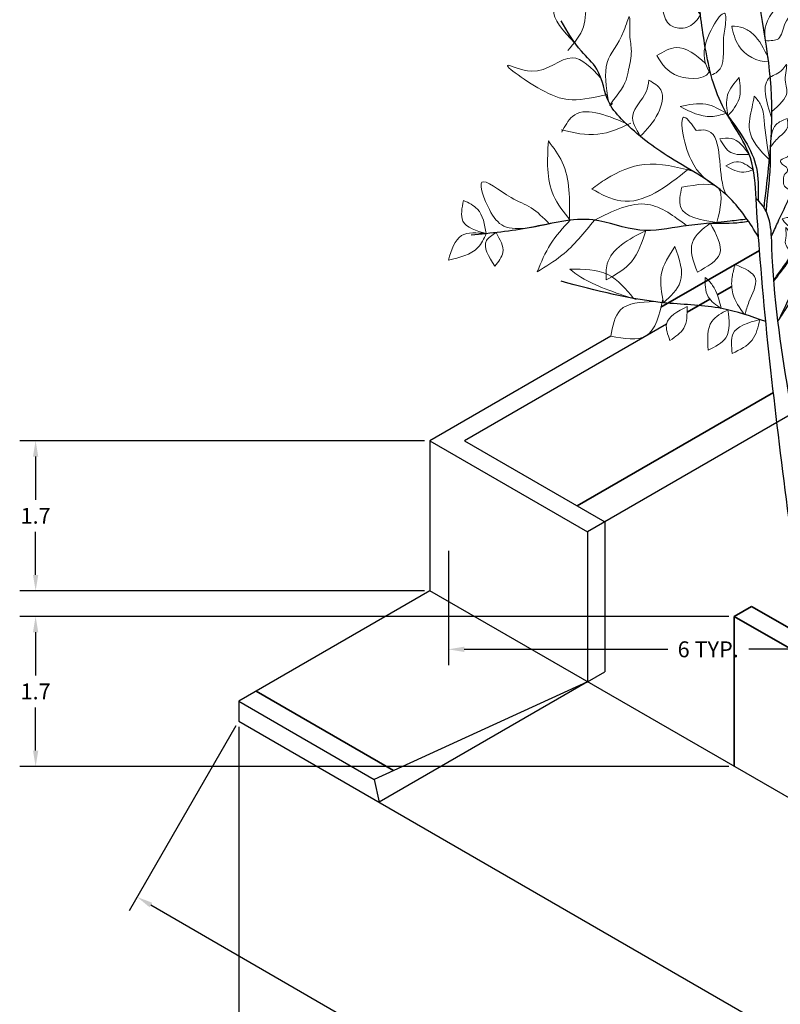
# Model space of a CAD drawing. Units: metres. Extents: x 12735 to 25554, y 20954 to 41989.
# Tile 2 of 15: x 12735.36 to 12743.97, y 20963.53 to 20974.68. Entities that reach past the tile are written whole.
import ezdxf

# ---------------------------------------------------------------- set-up
doc = ezdxf.new("R2010")
doc.units = ezdxf.units.M
doc.layers.get('Defpoints').update_dxf_attribs({"lineweight": 13})
for name, color, linetype, lineweight in [('A-ANNO-DIMS', 2, 'Continuous', 18), ('A-ELEV', 7, 'Continuous', 35), ('C-SITE', 8, 'Continuous', 25), ('TREES', 72, 'Continuous', 18)]:
    doc.layers.add(name, color=color, linetype=linetype, lineweight=lineweight)
doc.layers.add('STEM', color=32, linetype='Continuous')
doc.styles.get("Standard").update_dxf_attribs({"font": 'arial.ttf'})
doc.dimstyles.get("Standard").update_dxf_attribs({"dimtxt": 0.18, "dimasz": 0.18, "dimexe": 0.18, "dimexo": 0.0625, "dimgap": 0.09, "dimtad": 0, "dimtih": 1, "dimtoh": 1, "dimdec": 4, "dimzin": 0, "dimdsep": 46, "dimtxsty": 'Standard', "dimcen": 0.09, "dimadec": 0, "dimazin": 0, "dimtfac": 1, "dimtdec": 4, "dimtofl": 0, "dimtmove": 0, "dimatfit": 3, "dimfxl": 1, "dimtolj": 1, "dimtzin": 0, "dimarcsym": 0})

# ---------------------------------------------------------------- blocks, each defined once
blk = doc.blocks.new('TREES')
blk.add_line((12743.7, 20972.648), (12743.7, 20972.648))
at = {"layer": 'STEM'}
for points, knots in [([(12743.791, 20972.546), (12743.793, 20972.564), (12743.795, 20972.582), (12743.797, 20972.6), (12743.801, 20972.637), (12743.806, 20972.674), (12743.81, 20972.711), (12743.845, 20973.018), (12743.938, 20973.826), (12743.743, 20974.806), (12743.607, 20975.634), (12743.413, 20975.893), (12743.333, 20975.999)], [-0.164913, -0.164913, -0.164913, -0.164913, -0.110972, -0.110972, -0.110972, 0, 0, 0, 0.920963, 2.426088, 2.990404, 3.384799, 3.384799, 3.384799, 3.384799]), ([(12743.7, 20972.648), (12743.691, 20972.807), (12743.671, 20973.194), (12743.257, 20973.699), (12743.111, 20974.379), (12743.038, 20974.998), (12742.993, 20975.377), (12742.974, 20975.54)], [0, 0, 0, 0, 0.469346, 1.137622, 1.869488, 2.521439, 3.013071, 3.013071, 3.013071, 3.013071]), ([(12743.874, 20972.227), (12743.898, 20972.277), (12743.921, 20972.328), (12743.945, 20972.378), (12744.022, 20972.541), (12744.105, 20972.717), (12744.205, 20972.963), (12744.312, 20973.088), (12744.183, 20973.501), (12744.667, 20973.973), (12744.707, 20974.64), (12744.896, 20975.012), (12744.823, 20975.434), (12744.85, 20975.23), (12744.867, 20975.1)], [-0.166951, -0.166951, -0.166951, -0.166951, 0, 0, 0, 0.539768, 0.582066, 0.798222, 0.98781, 1.7696, 2.524754, 2.899414, 3.105113, 3.460848, 3.460848, 3.460848, 3.460848]), ([(12743.728, 20972.218), (12743.63, 20972.372), (12743.383, 20972.76), (12742.753, 20973.07), (12742.291, 20973.419), (12741.984, 20973.759), (12741.959, 20974.098), (12741.675, 20974.346), (12741.563, 20974.543), (12741.494, 20974.663)], [0, 0, 0, 0, 0.542161, 1.359078, 2.03444, 2.290187, 2.703676, 2.968549, 3.382864, 3.382864, 3.382864, 3.382864]), ([(12743.967, 20971.294), (12743.987, 20971.335), (12744.006, 20971.376), (12744.026, 20971.417), (12744.057, 20971.483), (12744.088, 20971.549), (12744.119, 20971.615), (12744.196, 20971.778), (12744.279, 20971.954), (12744.378, 20972.2), (12744.486, 20972.325), (12744.357, 20972.738), (12744.836, 20973.215), (12744.895, 20973.862), (12745.051, 20974.269), (12745.045, 20974.62), (12744.834, 20974.67), (12744.7, 20974.701)], [-0.355099, -0.355099, -0.355099, -0.355099, -0.218492, -0.218492, -0.218492, 0, 0, 0, 0.539768, 0.582066, 0.798222, 0.98781, 1.7696, 2.524754, 2.899414, 3.105113, 3.460848, 3.460848, 3.460848, 3.460848]), ([(12744.175, 20971.633), (12744.383, 20971.767), (12744.692, 20971.967), (12745.149, 20972.305), (12745.828, 20972.463), (12745.606, 20973.185), (12745.967, 20973.583), (12745.99, 20973.882), (12746.002, 20974.029)], [0, 0, 0, 0, 0.736164, 1.094646, 1.754618, 2.392389, 2.840214, 3.27091, 3.27091, 3.27091, 3.27091]), ([(12743.381, 20973.588), (12743.52, 20973.4), (12743.728, 20973.118), (12743.725, 20972.776), (12743.724, 20972.661), (12743.724, 20972.661), (12743.724, 20972.661), (12743.724, 20972.661), (12743.724, 20972.65), (12743.724, 20972.639), (12743.724, 20972.627)], [0, 0, 0, 0, 0.673099, 1.009429, 1.009429, 1.009429, 1.009429, 1.009429, 1.009429, 1.043412, 1.043412, 1.043412, 1.043412]), ([(12743.814, 20972.505), (12743.817, 20972.531), (12743.819, 20972.556), (12743.822, 20972.581), (12743.827, 20972.63), (12743.832, 20972.679), (12743.838, 20972.727), (12743.847, 20972.813), (12743.865, 20972.982), (12743.864, 20973.152), (12743.864, 20973.236)], [-0.2227932, -0.2227932, -0.2227932, -0.2227932, -0.1464713, -0.1464713, -0.1464713, 0, 0, 0, 0.2578951, 0.5103882, 0.5103882, 0.5103882, 0.5103882]), ([(12743.902, 20971.717), (12743.93, 20971.754), (12743.959, 20971.791), (12743.988, 20971.829), (12743.988, 20971.829), (12743.988, 20971.829), (12743.988, 20971.829), (12744.096, 20971.973), (12744.236, 20972.16), (12744.082, 20972.476), (12744.347, 20972.598), (12744.368, 20972.766), (12744.376, 20972.837)], [-0.129757, -0.129757, -0.129757, -0.129757, 0, 0, 0, 0, 0, 0, 0.485118, 0.62751, 0.913144, 1.120766, 1.120766, 1.120766, 1.120766]), ([(12744.111, 20968.725), (12743.967, 20969.837), (12743.799, 20971.142), (12743.712, 20972.453), (12743.7, 20972.648)], [0, 0, 0, 0, 3.359203, 3.944548, 3.944548, 3.944548, 3.944548]), ([(12744.332, 20968.825), (12744.189, 20969.936), (12743.871, 20971.161), (12743.872, 20972.51), (12743.7, 20972.648)], [0, 0, 0, 0, 3.359203, 3.972384, 3.972384, 3.972384, 3.972384]), ([(12743.597, 20972.418), (12743.533, 20972.41), (12743.292, 20972.379), (12742.889, 20972.351), (12742.364, 20972.241), (12741.803, 20972.489), (12741.157, 20972.302), (12740.698, 20972.258), (12740.474, 20972.237)], [0, 0, 0, 0, 0.193148, 0.727923, 1.218416, 1.762371, 2.471743, 3.152626, 3.152626, 3.152626, 3.152626]), ([(12743.181, 20972.372), (12743.296, 20972.37), (12743.441, 20972.368), (12743.583, 20972.39), (12743.613, 20972.395)], [0, 0, 0, 0, 0.3435042, 0.4329772, 0.4329772, 0.4329772, 0.4329772]), ([(12743.948, 20971.264), (12743.975, 20971.305), (12744.002, 20971.345), (12744.029, 20971.386), (12744.029, 20971.386), (12744.029, 20971.386), (12744.029, 20971.386), (12744.129, 20971.55), (12744.289, 20971.812), (12744.368, 20972.107), (12744.398, 20972.218)], [-0.148605, -0.148605, -0.148605, -0.148605, 0, 0, 0, 0, 0, 0, 0.572176, 0.914425, 0.914425, 0.914425, 0.914425]), ([(12743.901, 20971.729), (12743.929, 20971.768), (12743.958, 20971.808), (12743.986, 20971.847), (12743.986, 20971.847), (12743.986, 20971.847), (12743.986, 20971.847), (12744.02, 20971.892), (12744.062, 20971.951), (12744.099, 20972.014), (12744.107, 20972.028)], [-0.1467707, -0.1467707, -0.1467707, -0.1467707, 0, 0, 0, 0, 0, 0, 0.1684242, 0.2179474, 0.2179474, 0.2179474, 0.2179474]), ([(12743.81, 20971.258), (12743.646, 20971.316), (12743.283, 20971.443), (12742.486, 20971.453), (12741.888, 20971.61), (12741.494, 20971.714)], [0, 0, 0, 0, 0.519056, 1.146346, 2.366016, 2.366016, 2.366016, 2.366016])]:
    blk.add_open_spline(points, degree=3, knots=knots, dxfattribs=at)
blk.add_open_spline([(12744.644, 20971.941), (12744.672, 20971.961), (12744.701, 20971.98), (12744.73, 20972)], degree=3, dxfattribs=at)
at = {"layer": 'TREES'}
for points, knots in [([(12743.584, 20975.586), (12743.37, 20975.718), (12743.075, 20975.9), (12743.022, 20976.725), (12743.333, 20976.097), (12743.574, 20975.612)], [0, 0, 0, 0, 0.724771, 1.002271, 1.932196, 1.932196, 1.932196, 1.932196]), ([(12743.021, 20975.14), (12743.019, 20975.277), (12743.016, 20975.483), (12742.921, 20975.662), (12742.889, 20975.721)], [0, 0, 0, 0, 0.4023849, 0.6031293, 0.6031293, 0.6031293, 0.6031293]), ([(12743.021, 20975.14), (12742.985, 20975.224), (12742.928, 20975.356), (12742.766, 20975.539), (12742.854, 20975.638), (12742.901, 20975.69)], [0, 0, 0, 0, 0.2845416, 0.4465287, 0.6279758, 0.6279758, 0.6279758, 0.6279758]), ([(12743.718, 20974.979), (12743.671, 20975.164), (12743.598, 20975.454), (12743.323, 20975.534), (12743.223, 20975.563)], [0, 0, 0, 0, 0.519429, 0.8155501, 0.8155501, 0.8155501, 0.8155501]), ([(12743.223, 20975.563), (12743.266, 20975.448), (12743.36, 20975.195), (12743.592, 20975.055), (12743.718, 20974.979)], [0, 0, 0, 0, 0.3595778, 0.7860105, 0.7860105, 0.7860105, 0.7860105]), ([(12743.737, 20974.871), (12743.729, 20975.055), (12743.718, 20975.333), (12743.914, 20975.516), (12743.981, 20975.578)], [0, 0, 0, 0, 0.5134638, 0.7779111, 0.7779111, 0.7779111, 0.7779111]), ([(12743.737, 20974.871), (12743.801, 20974.971), (12743.939, 20975.186), (12743.966, 20975.441), (12743.981, 20975.578)], [0, 0, 0, 0, 0.351068, 0.7565079, 0.7565079, 0.7565079, 0.7565079]), ([(12741.648, 20974.411), (12741.519, 20974.547), (12741.281, 20974.798), (12741.642, 20974.995), (12741.673, 20975.511), (12741.684, 20975.149), (12741.787, 20975.033), (12741.768, 20974.824), (12741.781, 20974.575), (12741.641, 20974.411), (12741.569, 20974.326)], [0, 0, 0, 0, 0.446457, 0.821839, 1.096823, 1.294203, 1.491123, 1.594729, 1.894892, 2.216107, 2.216107, 2.216107, 2.216107]), ([(12743.031, 20975.058), (12743.048, 20975.139), (12743.077, 20975.281), (12743.184, 20975.377), (12743.231, 20975.418)], [0, 0, 0, 0, 0.2398723, 0.4207027, 0.4207027, 0.4207027, 0.4207027]), ([(12743.037, 20975.007), (12743.075, 20975.058), (12743.166, 20975.181), (12743.207, 20975.33), (12743.231, 20975.418)], [0, 0, 0, 0, 0.1895117, 0.457602, 0.457602, 0.457602, 0.457602]), ([(12744.796, 20974.806), (12744.757, 20974.909), (12744.688, 20975.088), (12744.514, 20975.28), (12744.523, 20975.414), (12744.526, 20975.464)], [0, 0, 0, 0, 0.3323117, 0.5782809, 0.7232611, 0.7232611, 0.7232611, 0.7232611]), ([(12744.805, 20974.813), (12744.804, 20974.918), (12744.803, 20975.076), (12744.822, 20975.37), (12744.643, 20975.427), (12744.526, 20975.464)], [0, 0, 0, 0, 0.3224266, 0.4885617, 0.8037384, 0.8037384, 0.8037384, 0.8037384]), ([(12743.07, 20974.733), (12742.98, 20974.863), (12742.848, 20975.053), (12742.433, 20975.446), (12742.649, 20974.915), (12742.651, 20974.573), (12742.961, 20974.576), (12743.034, 20974.678), (12743.071, 20974.73)], [0, 0, 0, 0, 0.54832, 0.799685, 1.166614, 1.565159, 1.742127, 1.925713, 1.925713, 1.925713, 1.925713]), ([(12744.796, 20974.806), (12744.882, 20974.878), (12745.017, 20974.992), (12745.211, 20975.15), (12745.228, 20975.277), (12745.236, 20975.337)], [0, 0, 0, 0, 0.3416822, 0.5370609, 0.7122352, 0.7122352, 0.7122352, 0.7122352]), ([(12744.839, 20974.951), (12744.859, 20975.055), (12744.903, 20975.272), (12745.122, 20975.315), (12745.236, 20975.337)], [0, 0, 0, 0, 0.2913456, 0.6064398, 0.6064398, 0.6064398, 0.6064398]), ([(12743.814, 20974.4), (12743.798, 20974.494), (12743.764, 20974.693), (12744.115, 20975.006), (12744.156, 20974.79), (12744.01, 20974.677), (12743.989, 20974.434), (12743.864, 20974.438), (12743.809, 20974.439)], [0, 0, 0, 0, 0.311146, 0.650746, 0.669061, 0.940573, 1.125337, 1.270427, 1.270427, 1.270427, 1.270427]), ([(12743.191, 20974.047), (12743.14, 20974.139), (12743.026, 20974.346), (12743.367, 20974.877), (12743.354, 20974.597), (12743.309, 20974.413), (12743.358, 20974.125), (12743.218, 20974.059), (12743.191, 20974.047)], [0, 0, 0, 0, 0.337622, 0.758697, 0.837919, 1.040495, 1.406258, 1.489574, 1.489574, 1.489574, 1.489574]), ([(12742.028, 20973.754), (12742.003, 20973.912), (12741.953, 20974.218), (12742.174, 20974.414), (12742.283, 20974.81), (12742.258, 20974.48), (12742.304, 20974.323), (12742.246, 20974.069), (12742.227, 20973.932), (12742.006, 20973.671), (12742.066, 20973.72), (12742.075, 20973.727)], [0, 0, 0, 0, 0.436736, 0.842969, 1.012738, 1.21393, 1.403734, 1.613178, 1.897283, 2.067562, 2.097274, 2.097274, 2.097274, 2.097274]), ([(12744.509, 20973.941), (12744.486, 20974.093), (12744.451, 20974.322), (12744.425, 20974.623), (12744.504, 20974.731), (12744.534, 20974.773)], [0, 0, 0, 0, 0.4681587, 0.7056034, 0.8580265, 0.8580265, 0.8580265, 0.8580265]), ([(12744.534, 20974.773), (12744.556, 20974.698), (12744.634, 20974.425), (12744.562, 20974.144), (12744.509, 20973.941)], [0, 0, 0, 0, 0.2327329, 0.8431329, 0.8431329, 0.8431329, 0.8431329]), ([(12744.554, 20973.975), (12744.669, 20974.016), (12744.893, 20974.094), (12745.019, 20974.421), (12745.06, 20974.624), (12745.08, 20974.72)], [0, 0, 0, 0, 0.348929, 0.678298, 0.9763146, 0.9763146, 0.9763146, 0.9763146]), ([(12743.835, 20974.249), (12743.789, 20974.346), (12743.724, 20974.484), (12743.556, 20974.594), (12743.468, 20974.601), (12743.424, 20974.604)], [0, 0, 0, 0, 0.3158223, 0.4463774, 0.5774617, 0.5774617, 0.5774617, 0.5774617]), ([(12743.424, 20974.604), (12743.442, 20974.527), (12743.487, 20974.324), (12743.715, 20974.191), (12743.841, 20974.206), (12743.841, 20974.206)], [0, 0, 0, 0, 0.2361186, 0.6165307, 0.6167763, 0.6167763, 0.6167763, 0.6167763]), ([(12744.618, 20974.118), (12744.717, 20974.268), (12744.844, 20974.462), (12745.022, 20974.606), (12745.062, 20974.638)], [0, 0, 0, 0, 0.5333846, 0.686651, 0.686651, 0.686651, 0.686651]), ([(12744.97, 20974.043), (12744.931, 20974.146), (12744.862, 20974.325), (12744.688, 20974.517), (12744.697, 20974.651), (12744.7, 20974.701)], [0, 0, 0, 0, 0.3323117, 0.5782809, 0.7232611, 0.7232611, 0.7232611, 0.7232611]), ([(12745.957, 20973.706), (12745.908, 20973.835), (12745.798, 20974.123), (12745.864, 20974.427), (12745.9, 20974.594)], [0, 0, 0, 0, 0.4051126, 0.906838, 0.906838, 0.906838, 0.906838]), ([(12745.9, 20974.594), (12745.955, 20974.471), (12746.037, 20974.287), (12746.01, 20974.092), (12746.002, 20974.029)], [0, 0, 0, 0, 0.3943838, 0.5836156, 0.5836156, 0.5836156, 0.5836156]), ([(12744.97, 20974.043), (12745.056, 20974.115), (12745.191, 20974.229), (12745.385, 20974.387), (12745.402, 20974.514), (12745.41, 20974.574)], [0, 0, 0, 0, 0.3416822, 0.5370609, 0.7122352, 0.7122352, 0.7122352, 0.7122352]), ([(12745.013, 20974.188), (12745.033, 20974.292), (12745.077, 20974.509), (12745.296, 20974.552), (12745.41, 20974.574)], [0, 0, 0, 0, 0.2913456, 0.6064398, 0.6064398, 0.6064398, 0.6064398]), ([(12743.128, 20974.182), (12743.019, 20974.275), (12742.841, 20974.427), (12742.65, 20974.313), (12742.577, 20974.27)], [0, 0, 0, 0, 0.3785086, 0.6144536, 0.6144536, 0.6144536, 0.6144536]), ([(12742.577, 20974.27), (12742.635, 20974.174), (12742.755, 20973.977), (12743.187, 20974.003), (12743.173, 20974.131), (12743.172, 20974.137)], [0, 0, 0, 0, 0.3386751, 0.6999446, 0.7185805, 0.7185805, 0.7185805, 0.7185805]), ([(12745.785, 20973.361), (12745.68, 20973.449), (12745.404, 20973.684), (12745.451, 20974.057), (12745.481, 20974.288)], [0, 0, 0, 0, 0.391493, 1.034106, 1.034106, 1.034106, 1.034106]), ([(12745.481, 20974.288), (12745.577, 20974.138), (12745.76, 20973.855), (12745.777, 20973.519), (12745.785, 20973.361)], [0, 0, 0, 0, 0.5245256, 0.9915723, 0.9915723, 0.9915723, 0.9915723]), ([(12741.943, 20974.016), (12741.835, 20974.13), (12741.594, 20974.382), (12741.272, 20973.991), (12740.687, 20974.27), (12741.289, 20973.836), (12741.63, 20973.742), (12741.878, 20973.799), (12742.016, 20973.831)], [0, 0, 0, 0, 0.397812, 0.88569, 1.156328, 1.66735, 1.991498, 2.394837, 2.394837, 2.394837, 2.394837]), ([(12743.879, 20973.555), (12743.816, 20973.752), (12743.731, 20974.021), (12743.982, 20974.067), (12744.068, 20974.224), (12744.006, 20973.984), (12744.093, 20973.824), (12743.961, 20973.709), (12743.879, 20973.638)], [0, 0, 0, 0, 0.469961, 0.638827, 0.705595, 0.853148, 1.022788, 1.296962, 1.296962, 1.296962, 1.296962]), ([(12744.356, 20973.647), (12744.309, 20973.708), (12744.202, 20973.846), (12744.245, 20974.018), (12744.268, 20974.113)], [0, 0, 0, 0, 0.2209277, 0.4981889, 0.4981889, 0.4981889, 0.4981889]), ([(12744.268, 20974.113), (12744.323, 20974.065), (12744.46, 20973.94), (12744.395, 20973.758), (12744.356, 20973.647)], [0, 0, 0, 0, 0.203616, 0.5174389, 0.5174389, 0.5174389, 0.5174389]), ([(12742.389, 20973.356), (12742.341, 20973.437), (12742.234, 20973.617), (12742.458, 20973.799), (12742.48, 20973.946), (12742.486, 20973.991)], [0, 0, 0, 0, 0.251735, 0.5591808, 0.6938707, 0.6938707, 0.6938707, 0.6938707]), ([(12742.486, 20973.991), (12742.542, 20973.959), (12742.68, 20973.88), (12742.598, 20973.572), (12742.464, 20973.433), (12742.389, 20973.356)], [0, 0, 0, 0, 0.1746142, 0.4385715, 0.7703441, 0.7703441, 0.7703441, 0.7703441]), ([(12743.381, 20973.588), (12743.369, 20973.67), (12743.344, 20973.833), (12743.453, 20973.958), (12743.508, 20974.02)], [0, 0, 0, 0, 0.2360196, 0.4713289, 0.4713289, 0.4713289, 0.4713289]), ([(12743.381, 20973.588), (12743.434, 20973.649), (12743.541, 20973.774), (12743.519, 20973.937), (12743.508, 20974.02)], [0, 0, 0, 0, 0.2309694, 0.4699481, 0.4699481, 0.4699481, 0.4699481]), ([(12744.683, 20973.178), (12744.66, 20973.33), (12744.625, 20973.559), (12744.599, 20973.86), (12744.677, 20973.968), (12744.708, 20974.01)], [0, 0, 0, 0, 0.4681587, 0.7056034, 0.8580265, 0.8580265, 0.8580265, 0.8580265]), ([(12744.708, 20974.01), (12744.73, 20973.935), (12744.807, 20973.662), (12744.735, 20973.381), (12744.683, 20973.178)], [0, 0, 0, 0, 0.2327329, 0.8431329, 0.8431329, 0.8431329, 0.8431329]), ([(12744.728, 20973.213), (12744.843, 20973.253), (12745.067, 20973.331), (12745.193, 20973.658), (12745.234, 20973.861), (12745.254, 20973.957)], [0, 0, 0, 0, 0.348929, 0.678298, 0.9763146, 0.9763146, 0.9763146, 0.9763146]), ([(12743.851, 20973.09), (12743.747, 20973.196), (12743.578, 20973.368), (12743.647, 20973.644), (12743.671, 20973.769), (12743.679, 20973.81)], [0, 0, 0, 0, 0.4076044, 0.6640272, 0.7921335, 0.7921335, 0.7921335, 0.7921335]), ([(12743.679, 20973.81), (12743.708, 20973.778), (12743.776, 20973.703), (12743.798, 20973.443), (12743.829, 20973.238), (12743.851, 20973.09)], [0, 0, 0, 0, 0.125659, 0.2981213, 0.7527794, 0.7527794, 0.7527794, 0.7527794]), ([(12744.792, 20973.355), (12744.891, 20973.505), (12745.018, 20973.699), (12745.196, 20973.843), (12745.236, 20973.876)], [0, 0, 0, 0, 0.5333846, 0.686651, 0.686651, 0.686651, 0.686651]), ([(12743.364, 20973.617), (12743.288, 20973.661), (12743.124, 20973.754), (12742.939, 20973.715), (12742.84, 20973.694)], [0, 0, 0, 0, 0.2535199, 0.5460217, 0.5460217, 0.5460217, 0.5460217]), ([(12742.221, 20973.506), (12741.989, 20973.602), (12741.674, 20973.731), (12741.536, 20973.471), (12741.5, 20973.404)], [0, 0, 0, 0, 0.6060397, 0.8197481, 0.8197481, 0.8197481, 0.8197481]), ([(12743.253, 20972.784), (12743.147, 20972.854), (12742.919, 20973.005), (12742.8, 20973.728), (12742.973, 20973.491), (12743.022, 20973.422)], [0, 0, 0, 0, 0.420416, 0.90702, 1.103207, 1.103207, 1.103207, 1.103207]), ([(12742.84, 20973.694), (12742.956, 20973.634), (12743.128, 20973.545), (12743.306, 20973.6), (12743.364, 20973.617)], [0, 0, 0, 0, 0.369417, 0.546183, 0.546183, 0.546183, 0.546183]), ([(12744.268, 20973.425), (12744.32, 20973.505), (12744.424, 20973.666), (12744.615, 20973.662), (12744.711, 20973.66)], [0, 0, 0, 0, 0.2669279, 0.5349854, 0.5349854, 0.5349854, 0.5349854]), ([(12744.268, 20973.425), (12744.336, 20973.433), (12744.51, 20973.454), (12744.635, 20973.582), (12744.711, 20973.66)], [0, 0, 0, 0, 0.1990667, 0.5143408, 0.5143408, 0.5143408, 0.5143408]), ([(12741.493, 20973.429), (12741.634, 20973.396), (12741.906, 20973.333), (12742.16, 20973.449), (12742.283, 20973.505)], [0, 0, 0, 0, 0.420024, 0.8136231, 0.8136231, 0.8136231, 0.8136231]), ([(12743.864, 20973.236), (12743.891, 20973.272), (12743.952, 20973.35), (12744.077, 20973.438), (12744.058, 20973.527), (12744.051, 20973.558)], [0, 0, 0, 0, 0.1377377, 0.3031534, 0.3935537, 0.3935537, 0.3935537, 0.3935537]), ([(12743.866, 20973.267), (12743.872, 20973.352), (12743.881, 20973.49), (12744.004, 20973.539), (12744.051, 20973.558)], [0, 0, 0, 0, 0.2295676, 0.3730638, 0.3730638, 0.3730638, 0.3730638]), ([(12743.022, 20973.422), (12743.059, 20973.426), (12743.334, 20973.456), (12743.256, 20972.956), (12743.349, 20972.723), (12743.36, 20972.696)], [0, 0, 0, 0, 0.1039343, 0.7792863, 0.8705393, 0.8705393, 0.8705393, 0.8705393]), ([(12745.697, 20972.996), (12745.547, 20972.999), (12745.238, 20973.004), (12745.268, 20973.314), (12745.283, 20973.473)], [0, 0, 0, 0, 0.3799868, 0.779071, 0.779071, 0.779071, 0.779071]), ([(12745.283, 20973.473), (12745.354, 20973.458), (12745.585, 20973.409), (12745.651, 20973.165), (12745.697, 20972.996)], [0, 0, 0, 0, 0.2074949, 0.6743984, 0.6743984, 0.6743984, 0.6743984]), ([(12741.595, 20972.406), (12741.523, 20972.496), (12741.318, 20972.752), (12741.336, 20973.087), (12741.348, 20973.304)], [0, 0, 0, 0, 0.3390919, 0.9589007, 0.9589007, 0.9589007, 0.9589007]), ([(12741.348, 20973.304), (12741.406, 20973.227), (12741.6, 20972.969), (12741.591, 20972.637), (12741.585, 20972.405)], [0, 0, 0, 0, 0.2865181, 0.9509807, 0.9509807, 0.9509807, 0.9509807]), ([(12743.621, 20973.151), (12743.561, 20973.233), (12743.473, 20973.354), (12743.333, 20973.334), (12743.288, 20973.327)], [0, 0, 0, 0, 0.2726158, 0.4022356, 0.4022356, 0.4022356, 0.4022356]), ([(12743.288, 20973.327), (12743.325, 20973.265), (12743.399, 20973.138), (12743.546, 20973.147), (12743.621, 20973.151)], [0, 0, 0, 0, 0.199886, 0.4070645, 0.4070645, 0.4070645, 0.4070645]), ([(12744.53, 20972.884), (12744.482, 20972.945), (12744.376, 20973.084), (12744.419, 20973.255), (12744.442, 20973.351)], [0, 0, 0, 0, 0.2209277, 0.4981889, 0.4981889, 0.4981889, 0.4981889]), ([(12744.442, 20973.351), (12744.496, 20973.302), (12744.634, 20973.177), (12744.569, 20972.995), (12744.53, 20972.884)], [0, 0, 0, 0, 0.203616, 0.5174389, 0.5174389, 0.5174389, 0.5174389]), ([(12745.697, 20972.996), (12745.724, 20973.08), (12745.77, 20973.226), (12745.915, 20973.262), (12745.976, 20973.277)], [0, 0, 0, 0, 0.2439478, 0.4222058, 0.4222058, 0.4222058, 0.4222058]), ([(12745.697, 20972.996), (12745.764, 20973.024), (12745.897, 20973.078), (12745.95, 20973.211), (12745.976, 20973.277)], [0, 0, 0, 0, 0.2073861, 0.4117039, 0.4117039, 0.4117039, 0.4117039]), ([(12744.074, 20972.655), (12744.086, 20972.673), (12744.124, 20972.731), (12743.998, 20972.782), (12744.014, 20972.867), (12744.011, 20972.925), (12744.052, 20972.944), (12744.07, 20973.015), (12743.988, 20973.027), (12743.97, 20973.091), (12744.03, 20973.11), (12744.072, 20973.132), (12744.097, 20973.169), (12744.133, 20973.163), (12744.172, 20973.164), (12744.216, 20973.136), (12744.296, 20973.17), (12744.282, 20973.105), (12744.259, 20973.057), (12744.341, 20973.048), (12744.328, 20972.986), (12744.32, 20972.935), (12744.299, 20972.884), (12744.258, 20972.852), (12744.236, 20972.821), (12744.215, 20972.805), (12744.179, 20972.793), (12744.139, 20972.807), (12744.095, 20972.746), (12744.111, 20972.739), (12744.111, 20972.739)], [0, 0, 0, 0, 0.055886, 0.185472, 0.25227, 0.305988, 0.338368, 0.378405, 0.48523, 0.4997, 0.565031, 0.618654, 0.656012, 0.680602, 0.71942, 0.77395, 0.836088, 0.890088, 0.913694, 0.979696, 1.032481, 1.0683, 1.142133, 1.186825, 1.224162, 1.25438, 1.26551, 1.333296, 1.383591, 1.385324, 1.385324, 1.385324, 1.385324]), ([(12742.983, 20972.961), (12742.799, 20973.009), (12742.463, 20973.098), (12742.071, 20972.928), (12741.893, 20972.798), (12741.839, 20972.759)], [0, 0, 0, 0, 0.553894, 1.01265, 1.215779, 1.215779, 1.215779, 1.215779]), ([(12743.669, 20972.977), (12743.606, 20973.025), (12743.504, 20973.102), (12743.398, 20973.043), (12743.358, 20973.021)], [0, 0, 0, 0, 0.2119595, 0.340544, 0.340544, 0.340544, 0.340544]), ([(12741.839, 20972.759), (12741.949, 20972.7), (12742.323, 20972.501), (12742.684, 20972.786), (12742.939, 20972.987)], [0, 0, 0, 0, 0.355589, 1.206871, 1.206871, 1.206871, 1.206871]), ([(12743.358, 20973.021), (12743.426, 20972.983), (12743.527, 20972.926), (12743.633, 20972.964), (12743.669, 20972.977)], [0, 0, 0, 0, 0.2166399, 0.3265492, 0.3265492, 0.3265492, 0.3265492]), ([(12745.681, 20972.634), (12745.776, 20972.643), (12745.97, 20972.661), (12746.056, 20972.838), (12746.1, 20972.929)], [0, 0, 0, 0, 0.2646598, 0.5464061, 0.5464061, 0.5464061, 0.5464061]), ([(12745.691, 20972.679), (12745.723, 20972.743), (12745.803, 20972.904), (12745.989, 20972.919), (12746.1, 20972.929)], [0, 0, 0, 0, 0.2025395, 0.5100625, 0.5100625, 0.5100625, 0.5100625]), ([(12741.358, 20972.366), (12741.291, 20972.434), (12741.162, 20972.564), (12740.909, 20972.646), (12740.492, 20972.989), (12740.719, 20972.381), (12740.905, 20972.253), (12741.437, 20972.382), (12741.361, 20972.366), (12741.358, 20972.366)], [0, 0, 0, 0, 0.274554, 0.529523, 0.902439, 1.220606, 1.740632, 1.953969, 1.962894, 1.962894, 1.962894, 1.962894]), ([(12742.858, 20972.779), (12743.034, 20972.81), (12743.375, 20972.87), (12743.295, 20972.539), (12743.257, 20972.379)], [0, 0, 0, 0, 0.4156133, 0.8046117, 0.8046117, 0.8046117, 0.8046117]), ([(12744.299, 20972.615), (12744.284, 20972.657), (12744.255, 20972.734), (12744.322, 20972.816), (12744.34, 20972.869), (12744.347, 20972.89)], [0, 0, 0, 0, 0.1248577, 0.2264879, 0.2926557, 0.2926557, 0.2926557, 0.2926557]), ([(12744.442, 20972.662), (12744.494, 20972.743), (12744.598, 20972.903), (12744.789, 20972.899), (12744.885, 20972.897)], [0, 0, 0, 0, 0.2669279, 0.5349854, 0.5349854, 0.5349854, 0.5349854]), ([(12744.442, 20972.662), (12744.51, 20972.671), (12744.684, 20972.691), (12744.809, 20972.819), (12744.885, 20972.897)], [0, 0, 0, 0, 0.1990667, 0.5143408, 0.5143408, 0.5143408, 0.5143408]), ([(12745.557, 20972.46), (12745.505, 20972.545), (12745.415, 20972.69), (12745.509, 20972.826), (12745.548, 20972.882)], [0, 0, 0, 0, 0.2672291, 0.4594629, 0.4594629, 0.4594629, 0.4594629]), ([(12745.548, 20972.882), (12745.623, 20972.785), (12745.735, 20972.639), (12745.619, 20972.519), (12745.581, 20972.479)], [0, 0, 0, 0, 0.3063433, 0.4579535, 0.4579535, 0.4579535, 0.4579535]), ([(12743.257, 20972.379), (12743.071, 20972.409), (12742.794, 20972.453), (12742.842, 20972.698), (12742.858, 20972.779)], [0, 0, 0, 0, 0.4478858, 0.6692237, 0.6692237, 0.6692237, 0.6692237]), ([(12744.14, 20972.455), (12744.129, 20972.498), (12744.112, 20972.571), (12744.173, 20972.643), (12744.195, 20972.684), (12744.204, 20972.7)], [0, 0, 0, 0, 0.124617, 0.2107396, 0.2658134, 0.2658134, 0.2658134, 0.2658134]), ([(12744.14, 20972.455), (12744.155, 20972.485), (12744.181, 20972.535), (12744.225, 20972.615), (12744.212, 20972.669), (12744.204, 20972.7)], [0, 0, 0, 0, 0.1037237, 0.1704768, 0.2630686, 0.2630686, 0.2630686, 0.2630686]), ([(12745.276, 20972.317), (12745.252, 20972.391), (12745.204, 20972.544), (12745.32, 20972.655), (12745.379, 20972.712)], [0, 0, 0, 0, 0.2148949, 0.4418034, 0.4418034, 0.4418034, 0.4418034]), ([(12745.276, 20972.317), (12745.329, 20972.378), (12745.429, 20972.493), (12745.395, 20972.642), (12745.379, 20972.712)], [0, 0, 0, 0, 0.2259484, 0.4304915, 0.4304915, 0.4304915, 0.4304915]), ([(12740.645, 20972.254), (12740.532, 20972.287), (12740.33, 20972.345), (12740.37, 20972.543), (12740.387, 20972.63)], [0, 0, 0, 0, 0.300298, 0.5327787, 0.5327787, 0.5327787, 0.5327787]), ([(12740.387, 20972.63), (12740.446, 20972.602), (12740.598, 20972.53), (12740.627, 20972.359), (12740.645, 20972.254)], [0, 0, 0, 0, 0.1847401, 0.4807235, 0.4807235, 0.4807235, 0.4807235]), ([(12742.916, 20972.343), (12742.772, 20972.452), (12742.448, 20972.697), (12742.076, 20972.511), (12741.869, 20972.407)], [0, 0, 0, 0, 0.501704, 1.133573, 1.133573, 1.133573, 1.133573]), ([(12744.192, 20972.515), (12744.244, 20972.502), (12744.335, 20972.479), (12744.372, 20972.56), (12744.387, 20972.593)], [0, 0, 0, 0, 0.1401829, 0.239855, 0.239855, 0.239855, 0.239855]), ([(12744.25, 20972.55), (12744.272, 20972.566), (12744.314, 20972.595), (12744.364, 20972.594), (12744.387, 20972.593)], [0, 0, 0, 0, 0.0790636, 0.1468534, 0.1468534, 0.1468534, 0.1468534]), ([(12744.137, 20972.378), (12744.147, 20972.414), (12744.168, 20972.49), (12744.249, 20972.485), (12744.292, 20972.483)], [0, 0, 0, 0, 0.0982704, 0.2114853, 0.2114853, 0.2114853, 0.2114853]), ([(12744.137, 20972.378), (12744.171, 20972.382), (12744.241, 20972.388), (12744.274, 20972.45), (12744.292, 20972.483)], [0, 0, 0, 0, 0.0955829, 0.1975677, 0.1975677, 0.1975677, 0.1975677]), ([(12744.868, 20972.097), (12744.937, 20972.148), (12745.072, 20972.246), (12745.072, 20972.413), (12745.073, 20972.494)], [0, 0, 0, 0, 0.2403434, 0.4714363, 0.4714363, 0.4714363, 0.4714363]), ([(12744.868, 20972.097), (12744.895, 20972.212), (12744.931, 20972.363), (12745.046, 20972.458), (12745.074, 20972.481)], [0, 0, 0, 0, 0.3374321, 0.4432568, 0.4432568, 0.4432568, 0.4432568]), ([(12745.582, 20972.481), (12745.667, 20972.516), (12745.814, 20972.576), (12745.958, 20972.516), (12746.019, 20972.491)], [0, 0, 0, 0, 0.2625898, 0.453199, 0.453199, 0.453199, 0.453199]), ([(12745.582, 20972.481), (12745.658, 20972.433), (12745.808, 20972.341), (12745.95, 20972.442), (12746.019, 20972.491)], [0, 0, 0, 0, 0.2451587, 0.4783488, 0.4783488, 0.4783488, 0.4783488]), ([(12741.223, 20971.823), (12741.319, 20971.881), (12741.571, 20972.033), (12741.755, 20972.264), (12741.869, 20972.407)], [0, 0, 0, 0, 0.3340001, 0.876507, 0.876507, 0.876507, 0.876507]), ([(12741.595, 20972.406), (12741.515, 20972.319), (12741.356, 20972.147), (12741.267, 20971.93), (12741.223, 20971.823)], [0, 0, 0, 0, 0.3521388, 0.6963584, 0.6963584, 0.6963584, 0.6963584]), ([(12743.181, 20972.372), (12743.094, 20972.305), (12742.907, 20972.162), (12742.991, 20971.938), (12743.035, 20971.819)], [0, 0, 0, 0, 0.2977969, 0.6372286, 0.6372286, 0.6372286, 0.6372286]), ([(12743.035, 20971.819), (12743.147, 20971.88), (12743.383, 20972.009), (12743.25, 20972.247), (12743.181, 20972.372)], [0, 0, 0, 0, 0.3275492, 0.688496, 0.688496, 0.688496, 0.688496]), ([(12744.145, 20972.348), (12744.132, 20972.384), (12744.105, 20972.455), (12744.032, 20972.434), (12743.996, 20972.423)], [0, 0, 0, 0, 0.098996, 0.196743, 0.196743, 0.196743, 0.196743]), ([(12743.996, 20972.423), (12744.027, 20972.377), (12744.069, 20972.315), (12744.13, 20972.341), (12744.146, 20972.347)], [0, 0, 0, 0, 0.1368513, 0.185287, 0.185287, 0.185287, 0.185287]), ([(12745.422, 20972.381), (12745.493, 20972.379), (12745.657, 20972.373), (12745.791, 20972.276), (12745.866, 20972.222)], [0, 0, 0, 0, 0.2087211, 0.4811791, 0.4811791, 0.4811791, 0.4811791]), ([(12745.422, 20972.381), (12745.521, 20972.247), (12745.661, 20972.058), (12745.82, 20972.185), (12745.866, 20972.222)], [0, 0, 0, 0, 0.3912381, 0.5526272, 0.5526272, 0.5526272, 0.5526272]), ([(12740.645, 20972.254), (12740.54, 20972.264), (12740.318, 20972.286), (12740.252, 20972.07), (12740.216, 20971.955)], [0, 0, 0, 0, 0.2808571, 0.5946199, 0.5946199, 0.5946199, 0.5946199]), ([(12740.216, 20971.955), (12740.344, 20971.984), (12740.536, 20972.026), (12740.618, 20972.197), (12740.645, 20972.254)], [0, 0, 0, 0, 0.3624795, 0.5464116, 0.5464116, 0.5464116, 0.5464116]), ([(12740.757, 20972.265), (12740.712, 20972.237), (12740.573, 20972.15), (12740.673, 20971.993), (12740.741, 20971.887)], [0, 0, 0, 0, 0.1417373, 0.4445248, 0.4445248, 0.4445248, 0.4445248]), ([(12740.741, 20971.887), (12740.783, 20971.937), (12740.878, 20972.054), (12740.801, 20972.189), (12740.757, 20972.265)], [0, 0, 0, 0, 0.1798963, 0.4162104, 0.4162104, 0.4162104, 0.4162104]), ([(12742.453, 20972.29), (12742.257, 20972.189), (12741.999, 20972.056), (12742.001, 20971.792), (12742.002, 20971.729)], [0, 0, 0, 0, 0.5792647, 0.7616052, 0.7616052, 0.7616052, 0.7616052]), ([(12742.002, 20971.729), (12742.108, 20971.788), (12742.333, 20971.914), (12742.411, 20972.161), (12742.453, 20972.29)], [0, 0, 0, 0, 0.3533474, 0.7448355, 0.7448355, 0.7448355, 0.7448355]), ([(12744.116, 20972.018), (12744.075, 20972.065), (12744.007, 20972.143), (12744.05, 20972.231), (12744.028, 20972.351), (12744.072, 20972.271), (12744.09, 20972.201), (12744.221, 20972.106), (12744.146, 20972.042), (12744.116, 20972.018)], [0, 0, 0, 0, 0.1633748, 0.2727914, 0.3326965, 0.376171, 0.4524353, 0.6040881, 0.701786, 0.701786, 0.701786, 0.701786]), ([(12744.746, 20972.012), (12744.742, 20972.047), (12744.733, 20972.118), (12744.771, 20972.218), (12744.826, 20972.252), (12744.849, 20972.268)], [0, 0, 0, 0, 0.1066556, 0.2131282, 0.2966333, 0.2966333, 0.2966333, 0.2966333]), ([(12744.746, 20972.012), (12744.773, 20972.045), (12744.822, 20972.105), (12744.891, 20972.268), (12744.848, 20972.268), (12744.847, 20972.268)], [0, 0, 0, 0, 0.1585708, 0.2833525, 0.285588, 0.285588, 0.285588, 0.285588]), ([(12745.053, 20972.215), (12745.111, 20972.233), (12745.273, 20972.284), (12745.353, 20972.117), (12745.405, 20972.009)], [0, 0, 0, 0, 0.1646898, 0.4645687, 0.4645687, 0.4645687, 0.4645687]), ([(12744.455, 20971.815), (12744.445, 20971.868), (12744.427, 20971.97), (12744.523, 20972.088), (12744.564, 20972.169), (12744.585, 20972.208)], [0, 0, 0, 0, 0.1538132, 0.2966411, 0.4292928, 0.4292928, 0.4292928, 0.4292928]), ([(12744.455, 20971.815), (12744.544, 20971.891), (12744.679, 20972.008), (12744.609, 20972.157), (12744.585, 20972.208)], [0, 0, 0, 0, 0.3019229, 0.4589929, 0.4589929, 0.4589929, 0.4589929]), ([(12745.053, 20972.215), (12745.087, 20972.171), (12745.174, 20972.057), (12745.317, 20972.027), (12745.405, 20972.009)], [0, 0, 0, 0, 0.1638697, 0.4194041, 0.4194041, 0.4194041, 0.4194041]), ([(12742.652, 20971.471), (12742.63, 20971.58), (12742.585, 20971.809), (12742.714, 20972.005), (12742.781, 20972.107)], [0, 0, 0, 0, 0.3207709, 0.6721329, 0.6721329, 0.6721329, 0.6721329]), ([(12742.652, 20971.471), (12742.732, 20971.545), (12742.92, 20971.718), (12742.832, 20971.965), (12742.781, 20972.107)], [0, 0, 0, 0, 0.3028446, 0.7080533, 0.7080533, 0.7080533, 0.7080533]), ([(12744.561, 20971.885), (12744.589, 20971.902), (12744.651, 20971.938), (12744.742, 20971.883), (12744.801, 20971.859), (12744.827, 20971.849)], [0, 0, 0, 0, 0.0920276, 0.2010844, 0.2860976, 0.2860976, 0.2860976, 0.2860976]), ([(12742.314, 20971.521), (12742.225, 20971.627), (12742.039, 20971.851), (12741.746, 20971.851), (12741.593, 20971.851)], [0, 0, 0, 0, 0.3968877, 0.8302181, 0.8302181, 0.8302181, 0.8302181]), ([(12741.593, 20971.851), (12741.666, 20971.793), (12741.821, 20971.668), (12742.447, 20971.471), (12742.312, 20971.521), (12742.311, 20971.521)], [0, 0, 0, 0, 0.3696351, 0.7965164, 0.7990281, 0.7990281, 0.7990281, 0.7990281]), ([(12743.566, 20971.341), (12743.514, 20971.414), (12743.424, 20971.54), (12743.418, 20971.749), (12743.449, 20971.857), (12743.463, 20971.904)], [0, 0, 0, 0, 0.2632417, 0.4527737, 0.6011812, 0.6011812, 0.6011812, 0.6011812]), ([(12743.463, 20971.904), (12743.567, 20971.861), (12743.772, 20971.775), (12743.623, 20971.516), (12743.587, 20971.385), (12743.574, 20971.338)], [0, 0, 0, 0, 0.2799093, 0.5517077, 0.7021324, 0.7021324, 0.7021324, 0.7021324]), ([(12744.561, 20971.885), (12744.599, 20971.871), (12744.674, 20971.844), (12744.795, 20971.792), (12744.822, 20971.84), (12744.827, 20971.849)], [0, 0, 0, 0, 0.1330667, 0.2587888, 0.2884885, 0.2884885, 0.2884885, 0.2884885]), ([(12743.304, 20971.408), (12743.247, 20971.446), (12743.157, 20971.505), (12743.12, 20971.647), (12743.123, 20971.722), (12743.125, 20971.759)], [0, 0, 0, 0, 0.196607, 0.3084716, 0.4203856, 0.4203856, 0.4203856, 0.4203856]), ([(12743.125, 20971.759), (12743.154, 20971.73), (12743.251, 20971.635), (12743.282, 20971.501), (12743.304, 20971.408)], [0, 0, 0, 0, 0.1222515, 0.400195, 0.400195, 0.400195, 0.400195]), ([(12742.056, 20971.092), (12742.207, 20971.066), (12742.53, 20971.009), (12742.604, 20971.335), (12742.644, 20971.51)], [0, 0, 0, 0, 0.3982442, 0.8534889, 0.8534889, 0.8534889, 0.8534889]), ([(12742.547, 20971.484), (12742.396, 20971.478), (12742.124, 20971.467), (12742.077, 20971.207), (12742.056, 20971.092)], [0, 0, 0, 0, 0.3960722, 0.7115037, 0.7115037, 0.7115037, 0.7115037]), ([(12742.918, 20971.429), (12742.811, 20971.373), (12742.636, 20971.282), (12742.7, 20971.111), (12742.725, 20971.045)], [0, 0, 0, 0, 0.3055467, 0.4944991, 0.4944991, 0.4944991, 0.4944991]), ([(12742.725, 20971.045), (12742.787, 20971.086), (12742.922, 20971.175), (12742.92, 20971.34), (12742.918, 20971.429)], [0, 0, 0, 0, 0.2088213, 0.4571427, 0.4571427, 0.4571427, 0.4571427]), ([(12743.381, 20971.391), (12743.311, 20971.354), (12743.137, 20971.26), (12743.15, 20971.056), (12743.158, 20970.935)], [0, 0, 0, 0, 0.2232821, 0.551466, 0.551466, 0.551466, 0.551466]), ([(12743.158, 20970.935), (12743.238, 20970.974), (12743.421, 20971.065), (12743.396, 20971.274), (12743.381, 20971.391)], [0, 0, 0, 0, 0.2445355, 0.5611675, 0.5611675, 0.5611675, 0.5611675]), ([(12743.743, 20971.282), (12743.611, 20971.245), (12743.396, 20971.185), (12743.421, 20970.978), (12743.431, 20970.898)], [0, 0, 0, 0, 0.3473993, 0.565418, 0.565418, 0.565418, 0.565418]), ([(12743.431, 20970.898), (12743.517, 20970.939), (12743.683, 20971.018), (12743.723, 20971.196), (12743.743, 20971.282)], [0, 0, 0, 0, 0.2699816, 0.5191769, 0.5191769, 0.5191769, 0.5191769])]:
    blk.add_open_spline(points, degree=3, knots=knots, dxfattribs=at)
blk.add_open_spline([(12744.347, 20972.89), (12744.357, 20972.872), (12744.367, 20972.854), (12744.376, 20972.837)], degree=3, dxfattribs=at)
blk = doc.blocks.new('*D6')
at = {"layer": 'A-ANNO-DIMS', "color": 0, "lineweight": -2, "transparency": 16777216}
for p, q in [((12740.216, 20968.663), (12740.216, 20967.367)), ((12746.1, 20968.663), (12746.1, 20967.367)), ((12740.396, 20967.547), (12742.7, 20967.547)), ((12745.92, 20967.547), (12743.617, 20967.547))]:
    blk.add_line(p, q, dxfattribs=at)
at = {"layer": 'A-ANNO-DIMS', "color": 0, "transparency": 16777216}
for points in [[(12740.396, 20967.577), (12740.396, 20967.517), (12740.216, 20967.547)], [(12745.92, 20967.577), (12745.92, 20967.517), (12746.1, 20967.547)]]:
    blk.add_solid(points, dxfattribs=at)
at = {"layer": 'Defpoints', "color": 0, "transparency": 16777216}
for p in [(12740.216, 20968.725), (12746.1, 20968.725), (12746.1, 20967.547)]:
    blk.add_point(p, dxfattribs=at)
at = {"layer": 'A-ANNO-DIMS', "color": 0, "transparency": 16777216, "insert": (12743.158, 20967.547), "char_height": 0.18, "attachment_point": 5}
blk.add_mtext('\\A1;6 TYP.', dxfattribs=at)
blk = doc.blocks.new('*D9')
at = {"layer": 'A-ANNO-DIMS', "color": 0, "lineweight": -2, "transparency": 16777216}
for p, q in [((12781.004, 20970.87), (12781.004, 20953.893)), ((12737.843, 20966.671), (12737.843, 20953.893)), ((12738.023, 20954.073), (12759.026, 20954.073)), ((12780.824, 20954.073), (12759.821, 20954.073))]:
    blk.add_line(p, q, dxfattribs=at)
at = {"layer": 'A-ANNO-DIMS', "color": 0, "transparency": 16777216}
for points in [[(12738.023, 20954.103), (12738.023, 20954.043), (12737.843, 20954.073)], [(12780.824, 20954.103), (12780.824, 20954.043), (12781.004, 20954.073)]]:
    blk.add_solid(points, dxfattribs=at)
at = {"layer": 'Defpoints', "color": 0, "transparency": 16777216}
for p in [(12781.004, 20970.933), (12737.843, 20966.733), (12781.004, 20954.073)]:
    blk.add_point(p, dxfattribs=at)
at = {"layer": 'A-ANNO-DIMS', "color": 0, "transparency": 16777216, "insert": (12759.423, 20954.073), "char_height": 0.18, "attachment_point": 5}
blk.add_mtext('\\A1;43.16', dxfattribs=at)
blk = doc.blocks.new('*D11')
at = {"layer": 'A-ANNO-DIMS', "color": 0, "lineweight": -2, "transparency": 16777216}
for p, q in [((12737.811, 20966.679), (12736.603, 20964.586)), ((12736.848, 20964.652), (12745.35, 20959.743)), ((12754.481, 20954.472), (12745.98, 20959.38)), ((12755.756, 20956.319), (12754.547, 20954.226))]:
    blk.add_line(p, q, dxfattribs=at)
at = {"layer": 'A-ANNO-DIMS', "color": 0, "transparency": 16777216}
for points in [[(12736.863, 20964.678), (12736.833, 20964.626), (12736.693, 20964.742)], [(12754.496, 20954.497), (12754.466, 20954.446), (12754.637, 20954.382)]]:
    blk.add_solid(points, dxfattribs=at)
at = {"layer": 'Defpoints', "color": 0, "transparency": 16777216}
for p in [(12737.843, 20966.733), (12736.693, 20964.742), (12755.787, 20956.373)]:
    blk.add_point(p, dxfattribs=at)
at = {"layer": 'A-ANNO-DIMS', "color": 0, "transparency": 16777216, "insert": (12745.665, 20959.562), "char_height": 0.18, "attachment_point": 5}
blk.add_mtext('\\A1;20.72', dxfattribs=at)
blk = doc.blocks.new('*D22')
at = {"layer": 'A-ANNO-DIMS', "color": 0, "lineweight": -2, "transparency": 16777216}
for p, q in [((12739.945, 20969.909), (12735.363, 20969.909)), ((12735.543, 20969.729), (12735.543, 20969.24)), ((12735.543, 20968.389), (12735.543, 20968.879)), ((12739.945, 20968.209), (12735.363, 20968.209))]:
    blk.add_line(p, q, dxfattribs=at)
at = {"layer": 'A-ANNO-DIMS', "color": 0, "transparency": 16777216}
for points in [[(12735.513, 20969.729), (12735.573, 20969.729), (12735.543, 20969.909)], [(12735.513, 20968.389), (12735.573, 20968.389), (12735.543, 20968.209)]]:
    blk.add_solid(points, dxfattribs=at)
at = {"layer": 'Defpoints', "color": 0, "transparency": 16777216}
for p in [(12740.008, 20969.909), (12735.543, 20968.209), (12740.008, 20968.209)]:
    blk.add_point(p, dxfattribs=at)
at = {"layer": 'A-ANNO-DIMS', "color": 0, "transparency": 16777216, "insert": (12735.543, 20969.059), "char_height": 0.18, "attachment_point": 5}
blk.add_mtext('\\A1;1.7', dxfattribs=at)
blk = doc.blocks.new('*D23')
at = {"layer": 'A-ANNO-DIMS', "color": 0, "lineweight": -2, "transparency": 16777216}
for p, q in [((12743.391, 20967.92), (12735.363, 20967.92)), ((12735.543, 20967.74), (12735.543, 20967.251)), ((12735.543, 20966.4), (12735.543, 20966.89)), ((12743.391, 20966.22), (12735.363, 20966.22))]:
    blk.add_line(p, q, dxfattribs=at)
at = {"layer": 'A-ANNO-DIMS', "color": 0, "transparency": 16777216}
for points in [[(12735.513, 20967.74), (12735.573, 20967.74), (12735.543, 20967.92)], [(12735.513, 20966.4), (12735.573, 20966.4), (12735.543, 20966.22)]]:
    blk.add_solid(points, dxfattribs=at)
at = {"layer": 'Defpoints', "color": 0, "transparency": 16777216}
for p in [(12743.453, 20967.92), (12735.543, 20966.22), (12743.453, 20966.22)]:
    blk.add_point(p, dxfattribs=at)
at = {"layer": 'A-ANNO-DIMS', "color": 0, "transparency": 16777216, "insert": (12735.543, 20967.07), "char_height": 0.18, "attachment_point": 5}
blk.add_mtext('\\A1;1.7', dxfattribs=at)

msp = doc.modelspace()

# ---------------------------------------------------------------- linework, layer by layer
at = {"layer": 'A-ELEV'}
for p, q in [((12743.7394, 20972.064), (12742.6231, 20971.4195)), ((12743.4243, 20971.6561), (12743.2613, 20971.562)), ((12743.1762, 20971.5128), (12742.9187, 20971.3642)), ((12743.896, 20970.4544), (12741.6756, 20969.1725)), ((12743.6488, 20968.0333), (12743.4531, 20967.9203)), ((12743.6488, 20968.0333), (12744.6014, 20967.4833)), ((12743.4531, 20967.9203), (12744.4057, 20967.3703)), ((12743.4531, 20967.9203), (12743.4531, 20966.2203)), ((12738.0383, 20967.0725), (12739.5946, 20966.174))]:
    msp.add_line(p, q, dxfattribs=at)
at = {"layer": 'C-SITE'}
for p, q in [((12748.4969, 20972.75), (12741.7923, 20968.8791)), ((12742.6863, 20971.23), (12740.3991, 20969.9095)), ((12742.0559, 20971.092), (12740.0077, 20969.9095)), ((12740.0077, 20969.9095), (12741.7923, 20968.8791)), ((12740.0077, 20969.9095), (12740.0077, 20968.2095)), ((12740.3991, 20969.9095), (12741.9881, 20968.9921)), ((12741.9881, 20968.9921), (12741.9881, 20967.2921)), ((12741.7923, 20968.8791), (12741.7923, 20967.1791)), ((12740.0077, 20968.2095), (12737.8426, 20966.9595)), ((12757.9519, 20957.8494), (12740.0077, 20968.2095)), ((12741.7923, 20967.1791), (12741.9881, 20967.2921)), ((12741.7923, 20967.1791), (12739.3762, 20966.0741)), ((12741.7923, 20967.1791), (12739.4316, 20965.8161)), ((12737.8426, 20966.9595), (12739.3762, 20966.0741)), ((12737.8426, 20966.9595), (12737.8426, 20966.7335)), ((12737.8426, 20966.7335), (12755.7869, 20956.3734)), ((12739.3762, 20966.0741), (12739.4316, 20965.8161))]:
    msp.add_line(p, q, dxfattribs=at)

# ---------------------------------------------------------------- block references
at = {"layer": 'TREES'}
msp.add_blockref('TREES', (0, 0), dxfattribs=at)

# ---------------------------------------------------------------- dimensions: what is measured, and where the dimension line sits
at = {"layer": 'A-ANNO-DIMS'}
dim = msp.add_linear_dim(base=(12781.0041, 20954.0734), p1=(12737.8426, 20966.7335), p2=(12781.0041, 20970.9326), dimstyle='Standard', override={"dimdec": 2, "dimlfac": 1, "dimrnd": 0, "dimzin": 0, "dimdsep": 46, "dimlunit": 2}, dxfattribs=at)
dim.commit()
dim.dimension.update_dxf_attribs({"geometry": '*D9', "text_midpoint": (12759.4234, 20954.0734)})
for base, p1, p2, angle, override, picture, middle in [((12735.5426, 20968.2095), (12740.0077, 20969.9095), (12740.0077, 20968.2095), 90, {"dimdec": 1, "dimlfac": 1, "dimrnd": 0, "dimzin": 0, "dimdsep": 46, "dimlunit": 2}, '*D22', (12735.5426, 20969.0595)), ((12735.5426, 20966.2203), (12743.4531, 20967.9203), (12743.4531, 20966.2203), 90, {"dimdec": 1, "dimlfac": 1, "dimrnd": 0, "dimzin": 0, "dimdsep": 46, "dimlunit": 2}, '*D23', (12735.5426, 20967.0703)), ((12736.6926, 20964.7416), (12755.7869, 20956.3734), (12737.8426, 20966.7335), 150, {"dimdec": 2, "dimlfac": 1, "dimrnd": 0, "dimzin": 0, "dimdsep": 46, "dimlunit": 2}, '*D11', (12745.6647, 20959.5616))]:
    dim = msp.add_linear_dim(base=base, p1=p1, p2=p2, angle=angle, dimstyle='Standard', override=override, dxfattribs=at)
    dim.commit()
    dim.dimension.update_dxf_attribs({"geometry": picture, "text_midpoint": middle})
dim = msp.add_linear_dim(base=(12746.1001, 20967.5471), p1=(12740.2163, 20968.7254), p2=(12746.1001, 20968.7254), text='<> TYP.', dimstyle='Standard', override={"dimdec": 0, "dimlfac": 1, "dimrnd": 0, "dimzin": 0, "dimdsep": 46, "dimlunit": 2}, dxfattribs=at)
dim.commit()
dim.dimension.update_dxf_attribs({"geometry": '*D6', "text_midpoint": (12743.1582, 20967.5471)})

doc.saveas('drawing.dxf')
